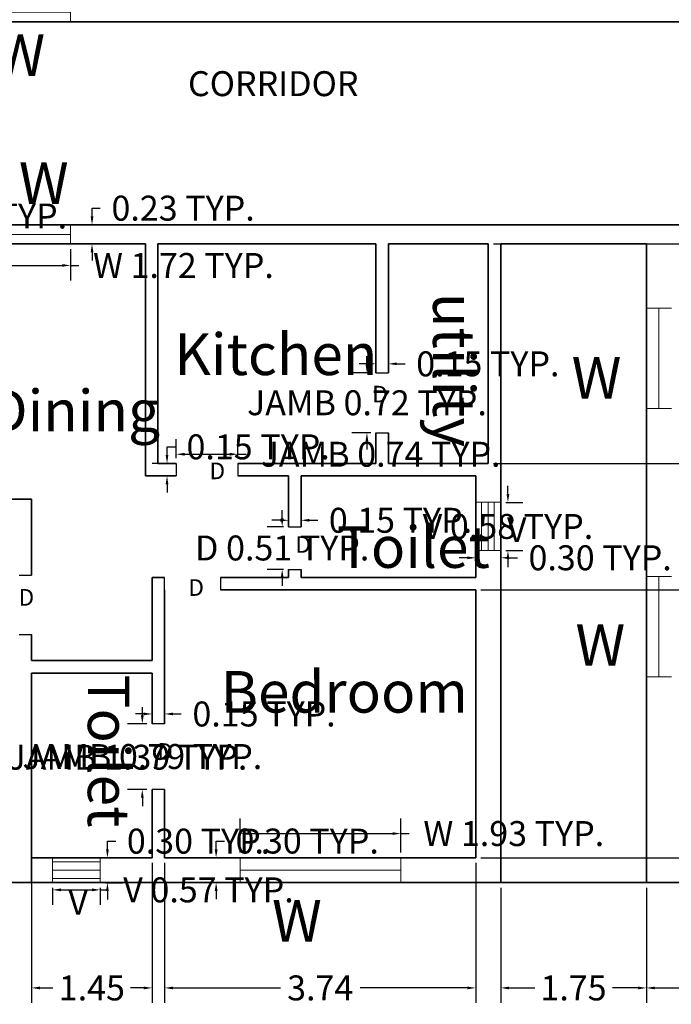
# Model space of a CAD drawing. Units: metres. Extents: x 11 to 49.6, y -23.3 to -0.8.
# Tile 2 of 5: x 17.9 to 25.8, y -23.3 to -11.5. Entities that reach past the tile are written whole.
import ezdxf

# ---------------------------------------------------------------- set-up
doc = ezdxf.new("R2010")
doc.units = ezdxf.units.M
doc.header["$MEASUREMENT"] = 0
for name, color, linetype, lineweight in [('A-ANNO-DIMS', 2, 'Continuous', 18), ('A-ANNO-IDEN', 3, 'Continuous', 18), ('A-AREA-IDEN', 7, 'Continuous', 18), ('A-DOOR', 3, 'Continuous', 25), ('A-GLAZ', 4, 'Continuous', 18), ('A-GLAZ-VENT', 4, 'Continuous', 18), ('A-WALL', 7, 'Continuous', 35)]:
    doc.layers.add(name, color=color, linetype=linetype, lineweight=lineweight)
doc.styles.get("Standard").update_dxf_attribs({"font": 'arial.ttf'})
doc.dimstyles.get("Standard").update_dxf_attribs({"dimtxt": 0.3, "dimasz": 0.1, "dimexe": 0.18, "dimexo": 0.0625, "dimgap": 0.09, "dimtad": 0, "dimtih": 1, "dimtoh": 1, "dimzin": 0, "dimdsep": 46, "dimtxsty": 'Standard', "dimcen": 0.09, "dimadec": 0, "dimazin": 0, "dimtfac": 1, "dimtofl": 0, "dimtmove": 0, "dimatfit": 3, "dimfxl": 1, "dimtolj": 1, "dimtzin": 0, "dimarcsym": 0})

# ---------------------------------------------------------------- blocks, each defined once
blk = doc.blocks.new('WIN-1207-D300')
for p, q in [((0.3, 1.207), (0, 1.207)), ((0.15, 1.207), (0.15, 0)), ((0, 0), (0.3, 0))]:
    blk.add_line(p, q)
blk = doc.blocks.new('WIN-1932-D300')
for p, q in [((0, 0.3), (0, 0)), ((1.932, 0.3), (1.932, 0)), ((1.932, 0.15), (1.932, 0.3)), ((0, 0.15), (1.932, 0.15))]:
    blk.add_line(p, q)
blk = doc.blocks.new('WIN-1724-D230')
for p, q in [((0, 0.23), (0, 0)), ((1.724, 0.23), (1.724, 0)), ((0, 0.115), (1.724, 0.115))]:
    blk.add_line(p, q)
blk = doc.blocks.new('VENT-572')
for p, q in [((0, 0.3), (0, 0)), ((0, 0.25), (0.572, 0.25)), ((0.572, 0.3), (0.572, 0)), ((0, 0.15), (0.572, 0.15)), ((0, 0.05), (0.572, 0.05))]:
    blk.add_line(p, q)
blk = doc.blocks.new('VENT-580')
for p, q in [((0, 0.58), (0.3, 0.58)), ((0.067, 0.58), (0.067, 0)), ((0.15, 0.58), (0.15, 0)), ((0.22, 0.58), (0.22, 0)), ((0, 0), (0.3, 0))]:
    blk.add_line(p, q)
blk = doc.blocks.new('DOOR-JAMB-741')
for p, q in [((0, 0.15), (0, 0)), ((0.741, 0.15), (0.741, 0))]:
    blk.add_line(p, q)
blk = doc.blocks.new('DOOR-JAMB-721')
for p, q in [((0, 0.721), (0.15, 0.721)), ((0, 0), (0.15, 0))]:
    blk.add_line(p, q)
blk = doc.blocks.new('DOOR-JAMB-513')
for p, q in [((0, 0.513), (0.15, 0.513)), ((0, 0), (0.15, 0))]:
    blk.add_line(p, q)
blk = doc.blocks.new('DOOR-JAMB-789')
for p, q in [((0.15, 0.789), (0, 0.789)), ((0.15, 0), (0, 0))]:
    blk.add_line(p, q)
blk = doc.blocks.new('*D30')
at = {"layer": 'A-ANNO-DIMS', "color": 0, "lineweight": -2, "transparency": 16777216}
for p, q in [((16.834, -14.229), (16.834, -14.605)), ((18.558, -14.229), (18.558, -14.605)), ((16.934, -14.425), (18.458, -14.425)), ((18.558, -14.425), (18.658, -14.425))]:
    blk.add_line(p, q, dxfattribs=at)
at = {"layer": 'A-ANNO-DIMS', "color": 0, "transparency": 16777216}
for points in [[(16.934, -14.408), (16.934, -14.441), (16.834, -14.425)], [(18.458, -14.408), (18.458, -14.441), (18.558, -14.425)]]:
    blk.add_solid(points, dxfattribs=at)
at = {"layer": 'Defpoints', "color": 0, "transparency": 16777216}
for p in [(16.834, -14.166), (18.558, -14.166), (18.558, -14.425)]:
    blk.add_point(p, dxfattribs=at)
at = {"layer": 'A-ANNO-DIMS', "color": 0, "transparency": 16777216, "insert": (19.915, -14.425), "char_height": 0.3, "attachment_point": 5}
blk.add_mtext('\\A1;W 1.72 TYP.', dxfattribs=at)
blk = doc.blocks.new('*D31')
at = {"layer": 'A-ANNO-DIMS', "color": 0, "lineweight": -2, "transparency": 16777216}
for p, q in [((18.816, -13.836), (18.816, -13.736)), ((18.816, -13.736), (18.916, -13.736)), ((18.62, -13.936), (18.996, -13.936)), ((18.62, -14.166), (18.996, -14.166)), ((18.816, -14.266), (18.816, -14.366))]:
    blk.add_line(p, q, dxfattribs=at)
at = {"layer": 'A-ANNO-DIMS', "color": 0, "transparency": 16777216}
for points in [[(18.8, -13.836), (18.833, -13.836), (18.816, -13.936)], [(18.8, -14.266), (18.833, -14.266), (18.816, -14.166)]]:
    blk.add_solid(points, dxfattribs=at)
at = {"layer": 'Defpoints', "color": 0, "transparency": 16777216}
for p in [(18.558, -13.936), (18.816, -13.936), (18.558, -14.166)]:
    blk.add_point(p, dxfattribs=at)
at = {"layer": 'A-ANNO-DIMS', "color": 0, "transparency": 16777216, "insert": (19.911, -13.736), "char_height": 0.3, "attachment_point": 5}
blk.add_mtext('\\A1;0.23 TYP.', dxfattribs=at)
blk = doc.blocks.new('*D32')
at = {"layer": 'A-ANNO-DIMS', "color": 0, "lineweight": -2, "transparency": 16777216}
for p, q in [((18.343, -21.91), (18.343, -22.113)), ((18.443, -21.933), (18.815, -21.933)), ((18.915, -21.91), (18.915, -22.113)), ((18.915, -21.933), (19.015, -21.933))]:
    blk.add_line(p, q, dxfattribs=at)
at = {"layer": 'A-ANNO-DIMS', "color": 0, "transparency": 16777216}
for points in [[(18.443, -21.916), (18.443, -21.95), (18.343, -21.933)], [(18.815, -21.916), (18.815, -21.95), (18.915, -21.933)]]:
    blk.add_solid(points, dxfattribs=at)
at = {"layer": 'Defpoints', "color": 0, "transparency": 16777216}
for p in [(18.343, -21.847), (18.915, -21.847), (18.915, -21.933)]:
    blk.add_point(p, dxfattribs=at)
at = {"layer": 'A-ANNO-DIMS', "color": 0, "transparency": 16777216, "insert": (20.216, -21.933), "char_height": 0.3, "attachment_point": 5}
blk.add_mtext('\\A1;V 0.57 TYP.', dxfattribs=at)
blk = doc.blocks.new('*D33')
at = {"layer": 'A-ANNO-DIMS', "color": 0, "lineweight": -2, "transparency": 16777216}
for p, q in [((19.001, -21.447), (19.001, -21.347)), ((19.001, -21.347), (19.101, -21.347)), ((18.978, -21.547), (19.181, -21.547)), ((18.978, -21.847), (19.181, -21.847)), ((19.001, -21.947), (19.001, -22.047))]:
    blk.add_line(p, q, dxfattribs=at)
at = {"layer": 'A-ANNO-DIMS', "color": 0, "transparency": 16777216}
for points in [[(18.985, -21.447), (19.018, -21.447), (19.001, -21.547)], [(18.985, -21.947), (19.018, -21.947), (19.001, -21.847)]]:
    blk.add_solid(points, dxfattribs=at)
at = {"layer": 'Defpoints', "color": 0, "transparency": 16777216}
for p in [(18.915, -21.547), (19.001, -21.547), (18.915, -21.847)]:
    blk.add_point(p, dxfattribs=at)
at = {"layer": 'A-ANNO-DIMS', "color": 0, "transparency": 16777216, "insert": (20.096, -21.347), "char_height": 0.3, "attachment_point": 5}
blk.add_mtext('\\A1;0.30 TYP.', dxfattribs=at)
blk = doc.blocks.new('*D38')
at = {"layer": 'A-ANNO-DIMS', "color": 0, "lineweight": -2, "transparency": 16777216}
for p, q in [((20.598, -21.484), (20.598, -21.076)), ((22.529, -21.484), (22.529, -21.076)), ((20.698, -21.256), (22.429, -21.256)), ((22.529, -21.256), (22.629, -21.256))]:
    blk.add_line(p, q, dxfattribs=at)
at = {"layer": 'A-ANNO-DIMS', "color": 0, "transparency": 16777216}
for points in [[(20.698, -21.24), (20.698, -21.273), (20.598, -21.256)], [(22.429, -21.24), (22.429, -21.273), (22.529, -21.256)]]:
    blk.add_solid(points, dxfattribs=at)
at = {"layer": 'Defpoints', "color": 0, "transparency": 16777216}
for p in [(22.529, -21.256), (20.598, -21.546), (22.529, -21.546)]:
    blk.add_point(p, dxfattribs=at)
at = {"layer": 'A-ANNO-DIMS', "color": 0, "transparency": 16777216, "insert": (23.886, -21.256), "char_height": 0.3, "attachment_point": 5}
blk.add_mtext('\\A1;W 1.93 TYP.', dxfattribs=at)
blk = doc.blocks.new('*D39')
at = {"layer": 'A-ANNO-DIMS', "color": 0, "lineweight": -2, "transparency": 16777216}
for p, q in [((20.308, -21.446), (20.308, -21.346)), ((20.308, -21.346), (20.408, -21.346)), ((20.535, -21.546), (20.128, -21.546)), ((20.535, -21.846), (20.128, -21.846)), ((20.308, -21.946), (20.308, -22.046))]:
    blk.add_line(p, q, dxfattribs=at)
at = {"layer": 'A-ANNO-DIMS', "color": 0, "transparency": 16777216}
for points in [[(20.291, -21.446), (20.325, -21.446), (20.308, -21.546)], [(20.291, -21.946), (20.325, -21.946), (20.308, -21.846)]]:
    blk.add_solid(points, dxfattribs=at)
at = {"layer": 'Defpoints', "color": 0, "transparency": 16777216}
for p in [(20.308, -21.546), (20.598, -21.546), (20.598, -21.846)]:
    blk.add_point(p, dxfattribs=at)
at = {"layer": 'A-ANNO-DIMS', "color": 0, "transparency": 16777216, "insert": (21.403, -21.346), "char_height": 0.3, "attachment_point": 5}
blk.add_mtext('\\A1;0.30 TYP.', dxfattribs=at)
blk = doc.blocks.new('*D40')
at = {"layer": 'A-ANNO-DIMS', "color": 0, "lineweight": -2, "transparency": 16777216}
for p, q in [((23.816, -17.174), (23.816, -17.074)), ((23.791, -17.274), (23.996, -17.274)), ((23.791, -17.853), (23.996, -17.853)), ((23.816, -17.953), (23.816, -18.053))]:
    blk.add_line(p, q, dxfattribs=at)
at = {"layer": 'A-ANNO-DIMS', "color": 0, "transparency": 16777216}
for points in [[(23.799, -17.174), (23.832, -17.174), (23.816, -17.274)], [(23.799, -17.953), (23.832, -17.953), (23.816, -17.853)]]:
    blk.add_solid(points, dxfattribs=at)
at = {"layer": 'Defpoints', "color": 0, "transparency": 16777216}
for p in [(23.729, -17.274), (23.816, -17.274), (23.729, -17.853)]:
    blk.add_point(p, dxfattribs=at)
at = {"layer": 'A-ANNO-DIMS', "color": 0, "transparency": 16777216, "insert": (23.816, -17.563), "char_height": 0.3, "attachment_point": 5}
blk.add_mtext('\\A1;V 0.58 TYP.', dxfattribs=at)
blk = doc.blocks.new('*D41')
at = {"layer": 'A-ANNO-DIMS', "color": 0, "lineweight": -2, "transparency": 16777216}
for p, q in [((23.329, -17.94), (23.229, -17.94)), ((23.429, -17.916), (23.429, -18.12)), ((23.729, -17.916), (23.729, -18.12)), ((23.829, -17.94), (23.929, -17.94))]:
    blk.add_line(p, q, dxfattribs=at)
at = {"layer": 'A-ANNO-DIMS', "color": 0, "transparency": 16777216}
for points in [[(23.329, -17.924), (23.329, -17.957), (23.429, -17.94)], [(23.829, -17.924), (23.829, -17.957), (23.729, -17.94)]]:
    blk.add_solid(points, dxfattribs=at)
at = {"layer": 'Defpoints', "color": 0, "transparency": 16777216}
for p in [(23.429, -17.853), (23.729, -17.853), (23.729, -17.94)]:
    blk.add_point(p, dxfattribs=at)
at = {"layer": 'A-ANNO-DIMS', "color": 0, "transparency": 16777216, "insert": (24.924, -17.94), "char_height": 0.3, "attachment_point": 5}
blk.add_mtext('\\A1;0.30 TYP.', dxfattribs=at)
blk = doc.blocks.new('*D42')
at = {"layer": 'A-ANNO-DIMS', "color": 0, "lineweight": -2, "transparency": 16777216}
for p, q in [((14.657, -13.874), (14.657, -13.65)), ((15.36, -13.874), (15.36, -13.65)), ((14.757, -13.83), (15.26, -13.83)), ((15.36, -13.83), (15.46, -13.83))]:
    blk.add_line(p, q, dxfattribs=at)
at = {"layer": 'A-ANNO-DIMS', "color": 0, "transparency": 16777216}
for points in [[(14.757, -13.814), (14.757, -13.847), (14.657, -13.83)], [(15.26, -13.814), (15.26, -13.847), (15.36, -13.83)]]:
    blk.add_solid(points, dxfattribs=at)
at = {"layer": 'Defpoints', "color": 0, "transparency": 16777216}
for p in [(15.36, -13.83), (14.657, -13.936), (15.36, -13.936)]:
    blk.add_point(p, dxfattribs=at)
at = {"layer": 'A-ANNO-DIMS', "color": 0, "transparency": 16777216, "insert": (17.075, -13.83), "char_height": 0.3, "attachment_point": 5}
blk.add_mtext('\\A1;JAMB 0.70 TYP.', dxfattribs=at)
blk = doc.blocks.new('*D44')
at = {"layer": 'A-ANNO-DIMS', "color": 0, "lineweight": -2, "transparency": 16777216}
for p, q in [((19.829, -16.744), (19.829, -16.515)), ((20.57, -16.744), (20.57, -16.515)), ((19.929, -16.695), (20.47, -16.695)), ((20.57, -16.695), (20.67, -16.695))]:
    blk.add_line(p, q, dxfattribs=at)
at = {"layer": 'A-ANNO-DIMS', "color": 0, "transparency": 16777216}
for points in [[(19.929, -16.678), (19.929, -16.712), (19.829, -16.695)], [(20.47, -16.678), (20.47, -16.712), (20.57, -16.695)]]:
    blk.add_solid(points, dxfattribs=at)
at = {"layer": 'Defpoints', "color": 0, "transparency": 16777216}
for p in [(19.829, -16.806), (20.57, -16.695), (20.57, -16.806)]:
    blk.add_point(p, dxfattribs=at)
at = {"layer": 'A-ANNO-DIMS', "color": 0, "transparency": 16777216, "insert": (22.285, -16.695), "char_height": 0.3, "attachment_point": 5}
blk.add_mtext('\\A1;JAMB 0.74 TYP.', dxfattribs=at)
blk = doc.blocks.new('*D45')
at = {"layer": 'A-ANNO-DIMS', "color": 0, "lineweight": -2, "transparency": 16777216}
for p, q in [((19.718, -16.706), (19.718, -16.606)), ((19.718, -16.606), (19.818, -16.606)), ((19.766, -16.806), (19.538, -16.806)), ((19.766, -16.956), (19.538, -16.956)), ((19.718, -17.056), (19.718, -17.156))]:
    blk.add_line(p, q, dxfattribs=at)
at = {"layer": 'A-ANNO-DIMS', "color": 0, "transparency": 16777216}
for points in [[(19.701, -16.706), (19.734, -16.706), (19.718, -16.806)], [(19.701, -17.056), (19.734, -17.056), (19.718, -16.956)]]:
    blk.add_solid(points, dxfattribs=at)
at = {"layer": 'Defpoints', "color": 0, "transparency": 16777216}
for p in [(19.718, -16.806), (19.829, -16.806), (19.829, -16.956)]:
    blk.add_point(p, dxfattribs=at)
at = {"layer": 'A-ANNO-DIMS', "color": 0, "transparency": 16777216, "insert": (20.813, -16.606), "char_height": 0.3, "attachment_point": 5}
blk.add_mtext('\\A1;0.15 TYP.', dxfattribs=at)
blk = doc.blocks.new('*D46')
at = {"layer": 'A-ANNO-DIMS', "color": 0, "lineweight": -2, "transparency": 16777216}
for p, q in [((22.121, -15.616), (22.121, -15.516)), ((22.166, -15.716), (21.941, -15.716)), ((22.166, -16.437), (21.941, -16.437)), ((22.121, -16.537), (22.121, -16.637))]:
    blk.add_line(p, q, dxfattribs=at)
at = {"layer": 'A-ANNO-DIMS', "color": 0, "transparency": 16777216}
for points in [[(22.104, -15.616), (22.137, -15.616), (22.121, -15.716)], [(22.104, -16.537), (22.137, -16.537), (22.121, -16.437)]]:
    blk.add_solid(points, dxfattribs=at)
at = {"layer": 'Defpoints', "color": 0, "transparency": 16777216}
for p in [(22.121, -15.716), (22.229, -15.716), (22.229, -16.437)]:
    blk.add_point(p, dxfattribs=at)
at = {"layer": 'A-ANNO-DIMS', "color": 0, "transparency": 16777216, "insert": (22.121, -16.076), "char_height": 0.3, "attachment_point": 5}
blk.add_mtext('\\A1;JAMB 0.72 TYP.', dxfattribs=at)
blk = doc.blocks.new('*D47')
at = {"layer": 'A-ANNO-DIMS', "color": 0, "lineweight": -2, "transparency": 16777216}
for p, q in [((22.229, -15.653), (22.229, -15.428)), ((22.379, -15.653), (22.379, -15.428)), ((22.129, -15.608), (22.029, -15.608)), ((22.479, -15.608), (22.579, -15.608))]:
    blk.add_line(p, q, dxfattribs=at)
at = {"layer": 'A-ANNO-DIMS', "color": 0, "transparency": 16777216}
for points in [[(22.129, -15.591), (22.129, -15.624), (22.229, -15.608)], [(22.479, -15.591), (22.479, -15.624), (22.379, -15.608)]]:
    blk.add_solid(points, dxfattribs=at)
at = {"layer": 'Defpoints', "color": 0, "transparency": 16777216}
for p in [(22.379, -15.608), (22.229, -15.716), (22.379, -15.716)]:
    blk.add_point(p, dxfattribs=at)
at = {"layer": 'A-ANNO-DIMS', "color": 0, "transparency": 16777216, "insert": (23.574, -15.608), "char_height": 0.3, "attachment_point": 5}
blk.add_mtext('\\A1;0.15 TYP.', dxfattribs=at)
blk = doc.blocks.new('*D48')
at = {"layer": 'A-ANNO-DIMS', "color": 0, "lineweight": -2, "transparency": 16777216}
for p, q in [((21.102, -17.466), (21.102, -17.366)), ((21.116, -17.566), (20.922, -17.566)), ((21.116, -18.079), (20.922, -18.079)), ((21.102, -18.179), (21.102, -18.279))]:
    blk.add_line(p, q, dxfattribs=at)
at = {"layer": 'A-ANNO-DIMS', "color": 0, "transparency": 16777216}
for points in [[(21.085, -17.466), (21.119, -17.466), (21.102, -17.566)], [(21.085, -18.179), (21.119, -18.179), (21.102, -18.079)]]:
    blk.add_solid(points, dxfattribs=at)
at = {"layer": 'Defpoints', "color": 0, "transparency": 16777216}
for p in [(21.102, -17.566), (21.179, -17.566), (21.179, -18.079)]:
    blk.add_point(p, dxfattribs=at)
at = {"layer": 'A-ANNO-DIMS', "color": 0, "transparency": 16777216, "insert": (21.102, -17.822), "char_height": 0.3, "attachment_point": 5}
blk.add_mtext('\\A1;D 0.51 TYP.', dxfattribs=at)
blk = doc.blocks.new('*D49')
at = {"layer": 'A-ANNO-DIMS', "color": 0, "lineweight": -2, "transparency": 16777216}
for p, q in [((21.179, -17.504), (21.179, -17.309)), ((21.329, -17.504), (21.329, -17.309)), ((21.079, -17.489), (20.979, -17.489)), ((21.429, -17.489), (21.529, -17.489))]:
    blk.add_line(p, q, dxfattribs=at)
at = {"layer": 'A-ANNO-DIMS', "color": 0, "transparency": 16777216}
for points in [[(21.079, -17.472), (21.079, -17.506), (21.179, -17.489)], [(21.429, -17.472), (21.429, -17.506), (21.329, -17.489)]]:
    blk.add_solid(points, dxfattribs=at)
at = {"layer": 'Defpoints', "color": 0, "transparency": 16777216}
for p in [(21.329, -17.489), (21.179, -17.566), (21.329, -17.566)]:
    blk.add_point(p, dxfattribs=at)
at = {"layer": 'A-ANNO-DIMS', "color": 0, "transparency": 16777216, "insert": (22.524, -17.489), "char_height": 0.3, "attachment_point": 5}
blk.add_mtext('\\A1;0.15 TYP.', dxfattribs=at)
blk = doc.blocks.new('*D50')
at = {"layer": 'A-ANNO-DIMS', "color": 0, "lineweight": -2, "transparency": 16777216}
for p, q in [((16.141, -20.484), (16.141, -20.158)), ((17.526, -20.484), (17.526, -20.158)), ((16.241, -20.338), (17.426, -20.338)), ((17.526, -20.338), (17.626, -20.338))]:
    blk.add_line(p, q, dxfattribs=at)
at = {"layer": 'A-ANNO-DIMS', "color": 0, "transparency": 16777216}
for points in [[(16.241, -20.321), (16.241, -20.355), (16.141, -20.338)], [(17.426, -20.321), (17.426, -20.355), (17.526, -20.338)]]:
    blk.add_solid(points, dxfattribs=at)
at = {"layer": 'Defpoints', "color": 0, "transparency": 16777216}
for p in [(17.526, -20.338), (16.141, -20.546), (17.526, -20.546)]:
    blk.add_point(p, dxfattribs=at)
at = {"layer": 'A-ANNO-DIMS', "color": 0, "transparency": 16777216, "insert": (19.242, -20.338), "char_height": 0.3, "attachment_point": 5}
blk.add_mtext('\\A1;JAMB 1.39 TYP.', dxfattribs=at)
blk = doc.blocks.new('*D52')
at = {"layer": 'A-ANNO-DIMS', "color": 0, "lineweight": -2, "transparency": 16777216}
for p, q in [((19.421, -19.836), (19.421, -19.736)), ((19.476, -19.936), (19.241, -19.936)), ((19.476, -20.725), (19.241, -20.725)), ((19.421, -20.825), (19.421, -20.925))]:
    blk.add_line(p, q, dxfattribs=at)
at = {"layer": 'A-ANNO-DIMS', "color": 0, "transparency": 16777216}
for points in [[(19.404, -19.836), (19.437, -19.836), (19.421, -19.936)], [(19.404, -20.825), (19.437, -20.825), (19.421, -20.725)]]:
    blk.add_solid(points, dxfattribs=at)
at = {"layer": 'Defpoints', "color": 0, "transparency": 16777216}
for p in [(19.421, -19.936), (19.539, -19.936), (19.539, -20.725)]:
    blk.add_point(p, dxfattribs=at)
at = {"layer": 'A-ANNO-DIMS', "color": 0, "transparency": 16777216, "insert": (19.421, -20.33), "char_height": 0.3, "attachment_point": 5}
blk.add_mtext('\\A1;JAMB 0.79 TYP.', dxfattribs=at)
blk = doc.blocks.new('*D53')
at = {"layer": 'A-ANNO-DIMS', "color": 0, "lineweight": -2, "transparency": 16777216}
for p, q in [((19.539, -19.874), (19.539, -19.638)), ((19.689, -19.874), (19.689, -19.638)), ((19.439, -19.818), (19.339, -19.818)), ((19.789, -19.818), (19.889, -19.818))]:
    blk.add_line(p, q, dxfattribs=at)
at = {"layer": 'A-ANNO-DIMS', "color": 0, "transparency": 16777216}
for points in [[(19.439, -19.801), (19.439, -19.834), (19.539, -19.818)], [(19.789, -19.801), (19.789, -19.834), (19.689, -19.818)]]:
    blk.add_solid(points, dxfattribs=at)
at = {"layer": 'Defpoints', "color": 0, "transparency": 16777216}
for p in [(19.689, -19.818), (19.539, -19.936), (19.689, -19.936)]:
    blk.add_point(p, dxfattribs=at)
at = {"layer": 'A-ANNO-DIMS', "color": 0, "transparency": 16777216, "insert": (20.884, -19.818), "char_height": 0.3, "attachment_point": 5}
blk.add_mtext('\\A1;0.15 TYP.', dxfattribs=at)
blk = doc.blocks.new('*D63')
at = {"layer": 'A-ANNO-DIMS', "color": 0, "lineweight": -2, "transparency": 16777216}
for p, q in [((23.729, -21.909), (23.729, -23.292)), ((25.48, -21.909), (25.48, -23.292)), ((23.829, -23.112), (24.138, -23.112)), ((25.38, -23.112), (25.071, -23.112))]:
    blk.add_line(p, q, dxfattribs=at)
at = {"layer": 'A-ANNO-DIMS', "color": 0, "transparency": 16777216}
for points in [[(23.829, -23.096), (23.829, -23.129), (23.729, -23.112)], [(25.38, -23.096), (25.38, -23.129), (25.48, -23.112)]]:
    blk.add_solid(points, dxfattribs=at)
at = {"layer": 'Defpoints', "color": 0, "transparency": 16777216}
for p in [(23.729, -21.846), (25.48, -21.846), (25.48, -23.112)]:
    blk.add_point(p, dxfattribs=at)
at = {"layer": 'A-ANNO-DIMS', "color": 0, "transparency": 16777216, "insert": (24.604, -23.112), "char_height": 0.3, "attachment_point": 5}
blk.add_mtext('\\A1;1.75', dxfattribs=at)
blk = doc.blocks.new('*D64')
at = {"layer": 'A-ANNO-DIMS', "color": 0, "lineweight": -2, "transparency": 16777216}
for p, q in [((25.48, -21.909), (25.48, -23.292)), ((35.309, -21.909), (35.309, -23.292)), ((25.58, -23.112), (29.915, -23.112)), ((35.209, -23.112), (30.874, -23.112))]:
    blk.add_line(p, q, dxfattribs=at)
at = {"layer": 'A-ANNO-DIMS', "color": 0, "transparency": 16777216}
for points in [[(25.58, -23.096), (25.58, -23.129), (25.48, -23.112)], [(35.209, -23.096), (35.209, -23.129), (35.309, -23.112)]]:
    blk.add_solid(points, dxfattribs=at)
at = {"layer": 'Defpoints', "color": 0, "transparency": 16777216}
for p in [(25.48, -21.846), (35.309, -21.846), (35.309, -23.112)]:
    blk.add_point(p, dxfattribs=at)
at = {"layer": 'A-ANNO-DIMS', "color": 0, "transparency": 16777216, "insert": (30.394, -23.112), "char_height": 0.3, "attachment_point": 5}
blk.add_mtext('\\A1;9.83', dxfattribs=at)
blk = doc.blocks.new('*D69')
at = {"layer": 'A-ANNO-DIMS', "color": 0, "lineweight": -2, "transparency": 16777216}
for p, q in [((18.089, -21.609), (18.089, -23.292)), ((19.539, -21.609), (19.539, -23.292)), ((18.189, -23.112), (18.347, -23.112)), ((19.439, -23.112), (19.28, -23.112))]:
    blk.add_line(p, q, dxfattribs=at)
at = {"layer": 'A-ANNO-DIMS', "color": 0, "transparency": 16777216}
for points in [[(18.189, -23.096), (18.189, -23.129), (18.089, -23.112)], [(19.439, -23.096), (19.439, -23.129), (19.539, -23.112)]]:
    blk.add_solid(points, dxfattribs=at)
at = {"layer": 'Defpoints', "color": 0, "transparency": 16777216}
for p in [(18.089, -21.546), (19.539, -21.546), (19.539, -23.112)]:
    blk.add_point(p, dxfattribs=at)
at = {"layer": 'A-ANNO-DIMS', "color": 0, "transparency": 16777216, "insert": (18.814, -23.112), "char_height": 0.3, "attachment_point": 5}
blk.add_mtext('\\A1;1.45', dxfattribs=at)
blk = doc.blocks.new('*D70')
at = {"layer": 'A-ANNO-DIMS', "color": 0, "lineweight": -2, "transparency": 16777216}
for p, q in [((19.689, -21.609), (19.689, -23.292)), ((23.429, -21.609), (23.429, -23.292)), ((19.789, -23.112), (21.08, -23.112)), ((23.329, -23.112), (22.038, -23.112))]:
    blk.add_line(p, q, dxfattribs=at)
at = {"layer": 'A-ANNO-DIMS', "color": 0, "transparency": 16777216}
for points in [[(19.789, -23.096), (19.789, -23.129), (19.689, -23.112)], [(23.329, -23.096), (23.329, -23.129), (23.429, -23.112)]]:
    blk.add_solid(points, dxfattribs=at)
at = {"layer": 'Defpoints', "color": 0, "transparency": 16777216}
for p in [(19.689, -21.546), (23.429, -21.546), (23.429, -23.112)]:
    blk.add_point(p, dxfattribs=at)
at = {"layer": 'A-ANNO-DIMS', "color": 0, "transparency": 16777216, "insert": (21.559, -23.112), "char_height": 0.3, "attachment_point": 5}
blk.add_mtext('\\A1;3.74', dxfattribs=at)
blk = doc.blocks.new('*D71')
at = {"layer": 'A-ANNO-DIMS', "color": 0, "lineweight": -2, "transparency": 16777216}
for p, q in [((23.641, -14.166), (36.754, -14.166)), ((36.574, -14.266), (36.574, -15.243)), ((36.574, -16.706), (36.574, -15.729)), ((23.641, -16.806), (36.754, -16.806))]:
    blk.add_line(p, q, dxfattribs=at)
at = {"layer": 'A-ANNO-DIMS', "color": 0, "transparency": 16777216}
for points in [[(36.558, -14.266), (36.591, -14.266), (36.574, -14.166)], [(36.558, -16.706), (36.591, -16.706), (36.574, -16.806)]]:
    blk.add_solid(points, dxfattribs=at)
at = {"layer": 'Defpoints', "color": 0, "transparency": 16777216}
for p in [(23.579, -14.166), (23.579, -16.806), (36.574, -16.806)]:
    blk.add_point(p, dxfattribs=at)
at = {"layer": 'A-ANNO-DIMS', "color": 0, "transparency": 16777216, "insert": (36.574, -15.486), "char_height": 0.3, "attachment_point": 5}
blk.add_mtext('\\A1;2.64', dxfattribs=at)
blk = doc.blocks.new('*D72')
at = {"layer": 'A-ANNO-DIMS', "color": 0, "lineweight": -2, "transparency": 16777216}
for p, q in [((23.491, -18.326), (36.754, -18.326)), ((36.574, -18.426), (36.574, -19.693)), ((36.574, -21.446), (36.574, -20.179)), ((23.491, -21.546), (36.754, -21.546))]:
    blk.add_line(p, q, dxfattribs=at)
at = {"layer": 'A-ANNO-DIMS', "color": 0, "transparency": 16777216}
for points in [[(36.558, -18.426), (36.591, -18.426), (36.574, -18.326)], [(36.558, -21.446), (36.591, -21.446), (36.574, -21.546)]]:
    blk.add_solid(points, dxfattribs=at)
at = {"layer": 'Defpoints', "color": 0, "transparency": 16777216}
for p in [(23.429, -18.326), (23.429, -21.546), (36.574, -21.546)]:
    blk.add_point(p, dxfattribs=at)
at = {"layer": 'A-ANNO-DIMS', "color": 0, "transparency": 16777216, "insert": (36.574, -19.936), "char_height": 0.3, "attachment_point": 5}
blk.add_mtext('\\A1;3.22', dxfattribs=at)

msp = doc.modelspace()

# ---------------------------------------------------------------- linework, layer by layer
at = {"layer": 'A-DOOR'}
for p, q in [((17.939, -18.147), (18.089, -18.147)), ((19.689, -18.326), (19.689, -18.176)), ((20.359, -18.176), (20.359, -18.326)), ((17.939, -18.863), (18.089, -18.863))]:
    msp.add_line(p, q, dxfattribs=at)
at = {"layer": 'A-WALL'}
for p, q in [((15.505, -11.496), (26.444, -11.496)), ((15.505, -11.496), (26.444, -11.496)), ((15.36, -13.936), (26.068, -13.936)), ((15.36, -13.936), (26.068, -13.936)), ((15.36, -14.166), (19.459, -14.166)), ((15.36, -14.166), (19.459, -14.166)), ((19.459, -16.806), (19.459, -14.166)), ((19.459, -16.956), (19.459, -14.166)), ((19.609, -16.806), (19.609, -14.166)), ((19.609, -14.166), (19.859, -14.166)), ((19.609, -14.166), (20.719, -14.166)), ((20.009, -14.166), (22.229, -14.166)), ((20.719, -14.166), (22.229, -14.166)), ((22.229, -15.716), (22.229, -14.166)), ((22.379, -14.166), (23.579, -14.166)), ((22.379, -14.166), (23.579, -14.166)), ((22.379, -15.716), (22.379, -14.166)), ((23.579, -16.806), (23.579, -14.166)), ((23.729, -21.846), (23.729, -14.166)), ((23.729, -14.166), (25.48, -14.166)), ((25.48, -21.846), (25.48, -14.166)), ((25.48, -14.166), (25.48, -21.846)), ((22.229, -16.806), (22.229, -16.437)), ((22.379, -16.806), (22.379, -16.437)), ((19.609, -16.806), (19.829, -16.806)), ((20.57, -16.806), (22.229, -16.806)), ((22.379, -16.806), (23.579, -16.806)), ((19.459, -16.956), (19.829, -16.956)), ((20.57, -16.956), (21.179, -16.956)), ((21.179, -17.566), (21.179, -16.956)), ((21.329, -16.956), (23.429, -16.956)), ((21.329, -17.566), (21.329, -16.956)), ((23.429, -18.176), (23.429, -16.956)), ((14.199, -17.236), (18.089, -17.236)), ((18.089, -18.147), (18.089, -17.236)), ((23.429, -18.176), (23.429, -17.926)), ((21.179, -18.176), (21.179, -18.079)), ((21.329, -18.176), (21.329, -18.079)), ((19.539, -18.176), (19.689, -18.176)), ((19.539, -19.176), (19.539, -18.176)), ((20.359, -18.176), (21.179, -18.176)), ((21.329, -18.176), (23.429, -18.176)), ((19.689, -19.936), (19.689, -18.326)), ((20.359, -18.326), (23.429, -18.326)), ((23.429, -21.546), (23.429, -18.326)), ((18.089, -19.176), (18.089, -18.863)), ((18.089, -19.176), (19.539, -19.176)), ((18.089, -19.326), (19.539, -19.326)), ((18.089, -21.846), (18.089, -19.326)), ((19.539, -19.376), (19.539, -19.326)), ((19.539, -19.936), (19.539, -19.326)), ((19.539, -21.546), (19.539, -20.725)), ((19.689, -21.546), (19.689, -20.725)), ((18.089, -21.546), (19.539, -21.546)), ((19.689, -21.546), (23.429, -21.546)), ((13.899, -21.846), (25.48, -21.846)), ((25.48, -21.846), (35.309, -21.846))]:
    msp.add_line(p, q, dxfattribs=at)

# ---------------------------------------------------------------- block references
at = {"layer": 'A-DOOR'}
for name, p in [('DOOR-JAMB-721', (22.229, -16.437)), ('DOOR-JAMB-741', (19.829, -16.956)), ('DOOR-JAMB-513', (21.179, -18.079)), ('DOOR-JAMB-789', (19.539, -20.725))]:
    msp.add_blockref(name, p, dxfattribs=at)
at = {"layer": 'A-GLAZ'}
for name, p in [('WIN-1724-D230', (16.834, -11.496)), ('WIN-1724-D230', (16.834, -14.166)), ('WIN-1932-D300', (20.598, -21.846))]:
    msp.add_blockref(name, p, dxfattribs=at)
at = {"layer": 'A-GLAZ', "rotation": 180}
for p in [(25.78, -14.939), (25.78, -18.165)]:
    msp.add_blockref('WIN-1207-D300', p, dxfattribs=at)
at = {"layer": 'A-GLAZ-VENT'}
for name, p in [('VENT-580', (23.429, -17.853)), ('VENT-572', (18.343, -21.847))]:
    msp.add_blockref(name, p, dxfattribs=at)

# ---------------------------------------------------------------- texts
at = {"layer": 'A-ANNO-IDEN', "attachment_point": 1}
for s, width, insert, char_height in [('W', 1.41386, (17.654, -11.645), 0.5), ('W', 1.41386, (17.937, -13.184), 0.5), ('W', 1.41386, (24.581, -15.526), 0.5), ('D', 0.77129, (22.184, -15.872), 0.2), ('D', 0.77129, (20.228, -16.795), 0.2), ('V', 0.1, (23.804, -17.452), 0.3), ('D', 0.77129, (21.26, -17.68), 0.2), ('D', 0.77129, (19.974, -18.198), 0.2), ('D', 0.77129, (17.933, -18.316), 0.2), ('W', 1.41386, (24.627, -18.739), 0.5), ('D', 0.77129, (19.6, -20.169), 0.2), ('V', 0.1, (18.531, -21.931), 0.3), ('W', 1.41386, (20.98, -22.055), 0.5)]:
    msp.add_mtext_dynamic_manual_height_columns(s, width=width, gutter_width=0.5, heights=[0], dxfattribs=dict(at, insert=insert, char_height=char_height))
at = {"layer": 'A-AREA-IDEN'}
for s, width, gutter_width, insert, char_height, attachment_point in [('CORRIDOR', 5.63863, 0.5, (19.97, -12.089), 0.3, 1), ('Kitchen', 2.63335, 1, (19.805, -15.243), 0.5, 1), ('Living/Dining', 2.63335, 1, (15.404, -16.421), 0.5, 7), ('Toilet', 2.63335, 1, (21.76, -18.061), 0.5, 7), ('Bedroom', 2.63335, 1, (20.363, -19.302), 0.5, 1)]:
    msp.add_mtext_dynamic_manual_height_columns(s, width=width, gutter_width=gutter_width, heights=[0], dxfattribs=dict(at, insert=insert, char_height=char_height, attachment_point=attachment_point))
at = {"layer": 'A-AREA-IDEN', "char_height": 0.5, "rotation": 270}
for s, insert, attachment_point in [('utility', (23.416, -14.755), 1), ('Toilet', (19.266, -21.182), 3)]:
    msp.add_mtext_dynamic_manual_height_columns(s, width=2.63335, gutter_width=1, heights=[0], dxfattribs=dict(at, insert=insert, attachment_point=attachment_point))

# ---------------------------------------------------------------- dimensions: what is measured, and where the dimension line sits
at = {"layer": 'A-ANNO-DIMS'}
for base, p1, p2, text, picture, middle in [((15.36, -13.83), (14.657, -13.936), (15.36, -13.936), 'JAMB <> TYP.', '*D42', (17.075, -13.83)), ((18.558, -14.425), (16.834, -14.166), (18.558, -14.166), 'W <> TYP.', '*D30', (19.915, -14.425)), ((22.379, -15.608), (22.229, -15.716), (22.379, -15.716), '<> TYP.', '*D47', (23.574, -15.608)), ((20.57, -16.695), (19.829, -16.806), (20.57, -16.806), 'JAMB <> TYP.', '*D44', (22.285, -16.695)), ((21.329, -17.489), (21.179, -17.566), (21.329, -17.566), '<> TYP.', '*D49', (22.524, -17.489)), ((23.729, -17.94), (23.429, -17.853), (23.729, -17.853), '<> TYP.', '*D41', (24.924, -17.94)), ((19.689, -19.818), (19.539, -19.936), (19.689, -19.936), '<> TYP.', '*D53', (20.884, -19.818)), ((17.5264, -20.3382), (16.1406, -20.546), (17.5264, -20.546), 'JAMB <> TYP.', '*D50', (19.2415, -20.3382)), ((22.529, -21.256), (20.598, -21.546), (22.529, -21.546), 'W <> TYP.', '*D38', (23.886, -21.256)), ((18.915, -21.933), (18.343, -21.847), (18.915, -21.847), 'V <> TYP.', '*D32', (20.216, -21.933))]:
    dim = msp.add_linear_dim(base=base, p1=p1, p2=p2, text=text, dimstyle='Standard', override={"dimdec": 2, "dimlfac": 1, "dimrnd": 0, "dimzin": 0, "dimdsep": 46, "dimlunit": 2}, dxfattribs=at)
    dim.commit()
    dim.dimension.update_dxf_attribs({"geometry": picture, "text_midpoint": middle})
for base, p1, p2, text, picture, middle in [((18.816, -13.936), (18.558, -14.166), (18.558, -13.936), '<> TYP.', '*D31', (19.911, -13.736)), ((22.121, -15.716), (22.229, -16.437), (22.229, -15.716), 'JAMB <> TYP.', '*D46', (22.121, -16.076)), ((19.718, -16.806), (19.829, -16.956), (19.829, -16.806), '<> TYP.', '*D45', (20.813, -16.606)), ((23.816, -17.274), (23.729, -17.853), (23.729, -17.274), 'V <> TYP.', '*D40', (23.816, -17.563)), ((21.102, -17.566), (21.179, -18.079), (21.179, -17.566), 'D <> TYP.', '*D48', (21.102, -17.822)), ((19.421, -19.936), (19.539, -20.725), (19.539, -19.936), 'JAMB <> TYP.', '*D52', (19.421, -20.33)), ((19.001, -21.547), (18.915, -21.847), (18.915, -21.547), '<> TYP.', '*D33', (20.096, -21.347)), ((20.308, -21.546), (20.598, -21.846), (20.598, -21.546), '<> TYP.', '*D39', (21.403, -21.346))]:
    dim = msp.add_linear_dim(base=base, p1=p1, p2=p2, angle=90, text=text, dimstyle='Standard', override={"dimdec": 2, "dimlfac": 1, "dimrnd": 0, "dimzin": 0, "dimdsep": 46, "dimlunit": 2}, dxfattribs=at)
    dim.commit()
    dim.dimension.update_dxf_attribs({"geometry": picture, "text_midpoint": middle})
for base, p1, p2, picture, middle in [((36.574, -16.806), (23.579, -14.166), (23.579, -16.806), '*D71', (36.574, -15.486)), ((36.574, -21.546), (23.429, -18.326), (23.429, -21.546), '*D72', (36.574, -19.936))]:
    dim = msp.add_linear_dim(base=base, p1=p1, p2=p2, angle=90, dimstyle='Standard', override={"dimdec": 2, "dimlfac": 1, "dimrnd": 0, "dimzin": 0, "dimdsep": 46, "dimlunit": 2}, dxfattribs=at)
    dim.commit()
    dim.dimension.update_dxf_attribs({"geometry": picture, "text_midpoint": middle})
for base, p1, p2, picture, middle in [((19.539, -23.112), (18.089, -21.546), (19.539, -21.546), '*D69', (18.814, -23.112)), ((23.429, -23.112), (19.689, -21.546), (23.429, -21.546), '*D70', (21.559, -23.112)), ((25.48, -23.112), (23.729, -21.846), (25.48, -21.846), '*D63', (24.604, -23.112)), ((35.309, -23.112), (25.48, -21.846), (35.309, -21.846), '*D64', (30.394, -23.112))]:
    dim = msp.add_linear_dim(base=base, p1=p1, p2=p2, dimstyle='Standard', override={"dimdec": 2, "dimlfac": 1, "dimrnd": 0, "dimzin": 0, "dimdsep": 46, "dimlunit": 2}, dxfattribs=at)
    dim.commit()
    dim.dimension.update_dxf_attribs({"geometry": picture, "text_midpoint": middle})

doc.saveas('drawing.dxf')
